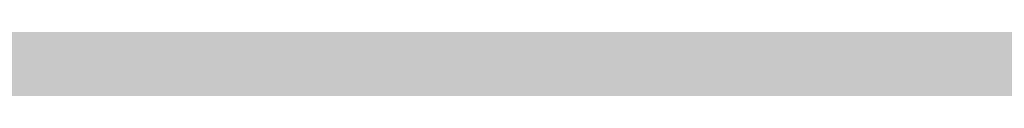
# Model space of a CAD drawing. Units: millimetres. Extents: x 0 to 2267, y 0 to 1823.
# Tile 126 of 256: x 1600.369 to 1605.705, y 1232.332 to 1232.602. Entities that reach past the tile are written whole.
import ezdxf

# ---------------------------------------------------------------- set-up
doc = ezdxf.new("R2010")
doc.units = ezdxf.units.MM
doc.header["$MEASUREMENT"] = 0
doc.layers.add('M-HATC', color=252, linetype='Continuous', lineweight=18)

msp = doc.modelspace()

# ---------------------------------------------------------------- hatches: boundary and pattern name
at = {"layer": 'M-HATC'}
h = msp.add_hatch(color=256, dxfattribs=at)
h.dxf.hatch_style = 1
h.paths.add_polyline_path([(2065.771, 1618.062, 0.236068), (2055.771, 1638.062), (1381.0868, 1638.062, 0.236068), (1371.0868, 1618.062), (1371.0868, 1603.062), (2055.771, 1603.062), (2065.771, 1603.062)])
h.paths.add_polyline_path([(2062.7718, 1550.2964), (2062.7718, 1560.2964), (1374.086, 1560.2964), (1374.086, 1550.2964), (1374.086, 1540.2964), (1384.086, 1540.2964), (1389.086, 1540.2964), (2062.7718, 1540.2964)])
h.paths.add_polyline_path([(1930.9289, 1282.7656), (1505.9289, 1282.7656), (1587.6276, 1235.5968, 0.131652), (1600.1276, 1232.2475), (1836.7302, 1232.2475, 0.131652), (1849.2302, 1235.5968)])
h.paths.add_polyline_path([(1930.9289, 1117.4171), (1905.9289, 1117.4171), (1505.9289, 1117.4171), (1505.9289, 1077.4171), (1930.9289, 1077.4171)])
h = msp.add_hatch(color=256, dxfattribs=at)
h.dxf.hatch_style = 1
h.paths.add_polyline_path([(2055.771, 1603.062), (1381.0868, 1603.062), (1381.0868, 1598.062), (2055.771, 1598.062)])
h.paths.add_polyline_path([(2055.771, 1598.062), (1381.0868, 1598.062), (1381.0868, 1593.062), (2055.771, 1593.062)])
h.paths.add_polyline_path([(2051.3074, 1536.7609), (1385.5504, 1536.7609), (1385.5504, 1526.7609), (1387.5504, 1526.7609), (1388.5366, 1525.0528), (1385.3319, 1521.2335), (1385.3319, 1521.2226), (2050.2542, 1522.7491), (2048.3212, 1525.0528), (2049.3074, 1526.7609), (2051.3074, 1526.7609)])
edge = h.paths.add_edge_path()
edge.add_arc((1847.5345, 1379.1492), 135, 222.603061, 222.890851, ccw=False)
edge.add_line((1748.1663, 1287.7656), (1683.0921, 1287.7656))
edge.add_arc((1583.7239, 1379.1492), 135, 317.109149, 317.396939, ccw=False)
edge.add_arc((1678.9686, 1290.6707), 5, 222.8909, 317.1091, ccw=False)
edge.add_arc((1774.2133, 1379.1492), 135, 222.603061, 222.890851, ccw=False)
edge.add_line((1674.8451, 1287.7656), (1609.7709, 1287.7656))
edge.add_arc((1510.4027, 1379.1492), 135, 317.109149, 317.396939, ccw=False)
edge.add_arc((1605.6474, 1290.6707), 5, 222.8909, 317.1091, ccw=False)
edge.add_arc((1700.8921, 1379.1492), 135, 222.603061, 222.890851, ccw=False)
edge.add_line((1601.5239, 1287.7656), (1536.4497, 1287.7656))
edge.add_arc((1437.0815, 1379.1492), 135, 317.109149, 317.396939, ccw=False)
edge.add_arc((1532.3262, 1290.6707), 5, 222.8909, 317.1091, ccw=False)
edge.add_arc((1627.5709, 1379.1492), 135, 222.603061, 222.890851, ccw=False)
edge.add_line((1528.2027, 1287.7656), (1505.9289, 1287.7656))
edge.add_spline(control_points=[(1505.9289, 1287.7656), (1504.2622, 1287.7656), (1504.2622, 1282.7656), (1505.9289, 1282.7656)], knot_values=[0, 0, 0, 0, 5, 5, 5, 5], degree=3, periodic=0)
edge.add_line((1505.9289, 1282.7656), (1930.9289, 1282.7656))
edge.add_spline(control_points=[(1930.9289, 1282.7656), (1932.5956, 1282.7656), (1932.5956, 1287.7656), (1930.9289, 1287.7656)], knot_values=[0, 0, 0, 0, 5, 5, 5, 5], degree=3, periodic=0)
edge.add_line((1930.9289, 1287.7656), (1903.0557, 1287.7656))
edge.add_arc((1803.6875, 1379.1492), 135, 317.109149, 317.396939, ccw=False)
edge.add_arc((1898.9322, 1290.6707), 5, 222.8909, 317.1091, ccw=False)
edge.add_arc((1994.1769, 1379.1492), 135, 222.603061, 222.890851, ccw=False)
edge.add_line((1894.8087, 1287.7656), (1829.7345, 1287.7656))
edge.add_arc((1730.3663, 1379.1492), 135, 317.109149, 317.396939, ccw=False)
edge.add_arc((1825.611, 1290.6707), 5, 222.8909, 317.1091, ccw=False)
edge.add_arc((1920.8557, 1379.1492), 135, 222.603061, 222.890851, ccw=False)
edge.add_line((1821.4875, 1287.7656), (1756.4133, 1287.7656))
edge.add_arc((1657.0451, 1379.1492), 135, 317.109149, 317.396939, ccw=False)
edge.add_arc((1752.2898, 1290.6707), 5, 222.8909, 317.1091, ccw=False)
edge = h.paths.add_edge_path()
edge.add_spline(control_points=[(1843.4289, 1227.2475), (1845.0956, 1227.2475), (1845.0956, 1232.2475), (1843.4289, 1232.2475)], knot_values=[0, 0, 0, 0, 5, 5, 5, 5], degree=3, periodic=0)
edge.add_line((1843.4289, 1232.2475), (1593.4289, 1232.2475))
edge.add_spline(control_points=[(1593.4289, 1232.2475), (1591.7622, 1232.2475), (1591.7622, 1227.2475), (1593.4289, 1227.2475)], knot_values=[0, 0, 0, 0, 5, 5, 5, 5], degree=3, periodic=0)
edge.add_line((1593.4289, 1227.2475), (1843.4289, 1227.2475))
h.paths.add_polyline_path([(1905.9289, 1127.4171), (1530.9289, 1127.4171, 0.414214), (1520.9289, 1117.4171), (1530.9289, 1117.4171), (1915.9289, 1117.4171, 0.414214)])
edge = h.paths.add_edge_path()
edge.add_arc((1397.0858, 1498.4078), 12.7299, 90.78215, 190.87871, ccw=False)
edge.add_line((1396.912, 1511.1365), (1428.0097, 1511.3488))
edge.add_line((1428.0097, 1511.3488), (1433.0097, 1511.3488))
edge.add_line((1433.0097, 1511.3488), (1434.439, 1511.3488))
edge.add_arc((1419.474, 1498.0804), 20, 41.561, 74.08211)
edge.add_line((1424.9592, 1517.3135), (1399.9351, 1517.2561))
edge.add_spline(control_points=[(1399.9307, 1517.2561), (1399.884, 1517.2131), (1399.8328, 1517.1689), (1399.7774, 1517.1236)], knot_values=[11.567499, 11.567499, 11.567499, 11.567499, 11.814249, 11.814249, 11.814249, 11.814249], degree=3, periodic=0)
edge.add_spline(control_points=[(1399.6328, 1517.0099), (1399.5831, 1516.9721), (1399.5307, 1516.9338), (1399.4759, 1516.8947)], knot_values=[11.167718, 11.167718, 11.167718, 11.167718, 11.365188, 11.365188, 11.365188, 11.365188], degree=3, periodic=0)
edge.add_spline(control_points=[(1399.3398, 1516.8001), (1399.1514, 1516.6719), (1398.9384, 1516.5377), (1398.704, 1516.3994)], knot_values=[10.376405, 10.376405, 10.376405, 10.376405, 11.00994, 11.00994, 11.00994, 11.00994], degree=3, periodic=0)
edge.add_spline(control_points=[(1398.6572, 1516.3719), (1398.5789, 1516.326), (1398.4983, 1516.2797), (1398.4155, 1516.2331)], knot_values=[10.125175, 10.125175, 10.125175, 10.125175, 10.334406, 10.334406, 10.334406, 10.334406], degree=3, periodic=0)
edge.add_spline(control_points=[(1398.2642, 1516.1487), (1398.196, 1516.1111), (1398.1263, 1516.0732), (1398.0555, 1516.0351)], knot_values=[9.832246, 9.832246, 9.832246, 9.832246, 9.999658, 9.999658, 9.999658, 9.999658], degree=3, periodic=0)
edge.add_spline(control_points=[(1397.9987, 1516.0048), (1397.7312, 1515.8621), (1397.446, 1515.7171), (1397.1466, 1515.5714)], knot_values=[9.161808, 9.161808, 9.161808, 9.161808, 9.787769, 9.787769, 9.787769, 9.787769], degree=3, periodic=0)
edge.add_spline(control_points=[(1397.1466, 1515.5714), (1396.8418, 1515.423), (1396.5222, 1515.274), (1396.1914, 1515.1262)], knot_values=[8.524455, 8.524455, 8.524455, 8.524455, 9.161808, 9.161808, 9.161808, 9.161808], degree=3, periodic=0)
edge.add_spline(control_points=[(1396.0777, 1515.0756), (1395.9854, 1515.0348), (1395.8922, 1514.994), (1395.7983, 1514.9534)], knot_values=[8.275193, 8.275193, 8.275193, 8.275193, 8.451726, 8.451726, 8.451726, 8.451726], degree=3, periodic=0)
edge.add_spline(control_points=[(1395.6018, 1514.8691), (1395.4997, 1514.8257), (1395.3968, 1514.7824), (1395.2932, 1514.7394)], knot_values=[7.962917, 7.962917, 7.962917, 7.962917, 8.152764, 8.152764, 8.152764, 8.152764], degree=3, periodic=0)
edge.add_spline(control_points=[(1395.2116, 1514.7057), (1394.8278, 1514.5475), (1394.4345, 1514.3929), (1394.0364, 1514.2442)], knot_values=[7.21254, 7.21254, 7.21254, 7.21254, 7.913148, 7.913148, 7.913148, 7.913148], degree=3, periodic=0)
edge.add_spline(control_points=[(1394.0364, 1514.2442), (1393.7076, 1514.1214), (1393.3754, 1514.0027), (1393.0427, 1513.8895)], knot_values=[6.633733, 6.633733, 6.633733, 6.633733, 7.21254, 7.21254, 7.21254, 7.21254], degree=3, periodic=0)
edge.add_spline(control_points=[(1392.8214, 1513.815), (1392.7198, 1513.7812), (1392.6181, 1513.7479), (1392.5166, 1513.7152)], knot_values=[6.328796, 6.328796, 6.328796, 6.328796, 6.505493, 6.505493, 6.505493, 6.505493], degree=3, periodic=0)
edge.add_spline(control_points=[(1392.5166, 1513.7152), (1392.3187, 1513.6515), (1392.1212, 1513.59), (1391.9244, 1513.531)], knot_values=[5.984605, 5.984605, 5.984605, 5.984605, 6.328796, 6.328796, 6.328796, 6.328796], degree=3, periodic=0)
edge.add_spline(control_points=[(1391.7915, 1513.4915), (1391.3122, 1513.3501), (1390.8384, 1513.2239), (1390.3784, 1513.1171)], knot_values=[5.066697, 5.066697, 5.066697, 5.066697, 5.907055, 5.907055, 5.907055, 5.907055], degree=3, periodic=0)
edge.add_spline(control_points=[(1390.3784, 1513.1171), (1390.1797, 1513.071), (1389.9836, 1513.0284), (1389.7907, 1512.9899)], knot_values=[4.70367, 4.70367, 4.70367, 4.70367, 5.066695, 5.066695, 5.066695, 5.066695], degree=3, periodic=0)
edge.add_spline(control_points=[(1389.422, 1512.9204), (1389.2459, 1512.8892), (1389.0729, 1512.8617), (1388.9036, 1512.8381)], knot_values=[4.130571, 4.130571, 4.130571, 4.130571, 4.469816, 4.469816, 4.469816, 4.469816], degree=3, periodic=0)
edge.add_spline(control_points=[(1388.9036, 1512.8381), (1388.591, 1512.7946), (1388.2911, 1512.7644), (1388.0071, 1512.7494)], knot_values=[3.504031, 3.504031, 3.504031, 3.504031, 4.130571, 4.130571, 4.130571, 4.130571], degree=3, periodic=0)
edge.add_spline(control_points=[(1387.9356, 1512.7459), (1387.8538, 1512.7423), (1387.7733, 1512.74), (1387.6944, 1512.739)], knot_values=[3.268866, 3.268866, 3.268866, 3.268866, 3.451164, 3.451164, 3.451164, 3.451164], degree=3, periodic=0)
edge.add_spline(control_points=[(1387.3351, 1512.7443), (1387.2076, 1512.7499), (1387.0847, 1512.7597), (1386.967, 1512.7739)], knot_values=[2.670686, 2.670686, 2.670686, 2.670686, 2.984, 2.984, 2.984, 2.984], degree=3, periodic=0)
edge.add_spline(control_points=[(1386.8327, 1512.7922), (1386.8209, 1512.7941), (1386.8092, 1512.7959), (1386.7975, 1512.7979)], knot_values=[2.516981, 2.516981, 2.516981, 2.516981, 2.549528, 2.549528, 2.549528, 2.549528], degree=3, periodic=0)
edge.add_spline(control_points=[(1386.4526, 1512.8735), (1386.4257, 1512.881), (1386.3993, 1512.889), (1386.3733, 1512.8972)], knot_values=[2.095869, 2.095869, 2.095869, 2.095869, 2.17941, 2.17941, 2.17941, 2.17941], degree=3, periodic=0)
edge.add_spline(control_points=[(1386.0691, 1513.0189), (1386.0634, 1513.0217), (1386.0577, 1513.0246), (1386.052, 1513.0275)], knot_values=[1.72453, 1.72453, 1.72453, 1.72453, 1.745933, 1.745933, 1.745933, 1.745933], degree=3, periodic=0)
edge.add_arc((1399.474, 1498.0804), 20, 131.82432, 180)
edge.add_arc((1630.3336, 1505.5484), 250.9708, 181.705176, 236.427975)
edge.add_arc((1605.3399, 1483.3044), 218.7822, 238.660829, 243.34961)
edge.add_arc((1647.0911, 1510.3592), 262.8986, 183.129836, 237.853442, ccw=False)
h.paths.add_polyline_path([(1406.5369, 1391.9644, 0.149382), (1491.5506, 1296.4418, -0.129517)], flags=17)
edge = h.paths.add_edge_path()
edge.add_arc((2037.3838, 1498.0804), 20, 0, 48.26587)
edge.add_spline(control_points=[(2050.6973, 1513.0052), (2050.6512, 1512.9847), (2050.6034, 1512.9655), (2050.5539, 1512.9477)], knot_values=[1.835652, 1.835652, 1.835652, 1.835652, 2.000781, 2.000781, 2.000781, 2.000781], degree=3, periodic=0)
edge.add_spline(control_points=[(2050.4616, 1512.9166), (2050.479, 1512.9221), (2050.4963, 1512.9277), (2050.5133, 1512.9335)], knot_values=[2.045477, 2.045477, 2.045477, 2.045477, 2.101389, 2.101389, 2.101389, 2.101389], degree=3, periodic=0)
edge.add_spline(control_points=[(2050.129, 1512.8342), (2050.1984, 1512.8473), (2050.2657, 1512.8623), (2050.3308, 1512.8792)], knot_values=[2.237629, 2.237629, 2.237629, 2.237629, 2.435841, 2.435841, 2.435841, 2.435841], degree=3, periodic=0)
edge.add_spline(control_points=[(2050.0946, 1512.8278), (2050.1061, 1512.8299), (2050.1176, 1512.832), (2050.129, 1512.8342)], knot_values=[2.435841, 2.435841, 2.435841, 2.435841, 2.468321, 2.468321, 2.468321, 2.468321], degree=3, periodic=0)
edge.add_spline(control_points=[(2049.7843, 1512.7851), (2049.8552, 1512.7922), (2049.9243, 1512.8008), (2049.9917, 1512.8109)], knot_values=[2.563852, 2.563852, 2.563852, 2.563852, 2.748541, 2.748541, 2.748541, 2.748541], degree=3, periodic=0)
edge.add_spline(control_points=[(2049.4052, 1512.7617), (2049.5364, 1512.7653), (2049.6629, 1512.773), (2049.7843, 1512.7851)], knot_values=[2.748541, 2.748541, 2.748541, 2.748541, 3.064882, 3.064882, 3.064882, 3.064882], degree=3, periodic=0)
edge.add_spline(control_points=[(2049.1698, 1512.7597), (2049.2336, 1512.7591), (2049.2965, 1512.7594), (2049.3584, 1512.7606)], knot_values=[3.102309, 3.102309, 3.102309, 3.102309, 3.2503, 3.2503, 3.2503, 3.2503], degree=3, periodic=0)
edge.add_spline(control_points=[(2048.8573, 1512.7691), (2048.9638, 1512.7638), (2049.068, 1512.7606), (2049.1698, 1512.7597)], knot_values=[3.2503, 3.2503, 3.2503, 3.2503, 3.486069, 3.486069, 3.486069, 3.486069], degree=3, periodic=0)
edge.add_spline(control_points=[(2048.6924, 1512.7789), (2048.3729, 1512.8009), (2048.0345, 1512.8411), (2047.6817, 1512.897)], knot_values=[3.606429, 3.606429, 3.606429, 3.606429, 4.2989, 4.2989, 4.2989, 4.2989], degree=3, periodic=0)
edge.add_spline(control_points=[(2047.6817, 1512.897), (2047.5458, 1512.9185), (2047.4077, 1512.9424), (2047.2678, 1512.9685)], knot_values=[4.2989, 4.2989, 4.2989, 4.2989, 4.565769, 4.565769, 4.565769, 4.565769], degree=3, periodic=0)
edge.add_spline(control_points=[(2047.2678, 1512.9685), (2047.1449, 1512.9914), (2047.0207, 1513.016), (2046.8951, 1513.0422)], knot_values=[4.565769, 4.565769, 4.565769, 4.565769, 4.799971, 4.799971, 4.799971, 4.799971], degree=3, periodic=0)
edge.add_spline(control_points=[(2046.8951, 1513.0422), (2046.5286, 1513.1188), (2046.1513, 1513.209), (2045.7676, 1513.3107)], knot_values=[4.799971, 4.799971, 4.799971, 4.799971, 5.483718, 5.483718, 5.483718, 5.483718], degree=3, periodic=0)
edge.add_spline(control_points=[(2045.7676, 1513.3107), (2045.3724, 1513.4154), (2044.9704, 1513.5322), (2044.5662, 1513.6588)], knot_values=[5.483718, 5.483718, 5.483718, 5.483718, 6.187866, 6.187866, 6.187866, 6.187866], degree=3, periodic=0)
edge.add_spline(control_points=[(2044.5662, 1513.6588), (2044.4149, 1513.7061), (2044.2633, 1513.7549), (2044.1116, 1513.8048)], knot_values=[6.187866, 6.187866, 6.187866, 6.187866, 6.451551, 6.451551, 6.451551, 6.451551], degree=3, periodic=0)
edge.add_spline(control_points=[(2044.1116, 1513.8048), (2043.9967, 1513.8427), (2043.8817, 1513.8813), (2043.7668, 1513.9205)], knot_values=[6.451551, 6.451551, 6.451551, 6.451551, 6.651434, 6.651434, 6.651434, 6.651434], degree=3, periodic=0)
edge.add_spline(control_points=[(2043.7668, 1513.9205), (2043.3716, 1514.0554), (2042.9774, 1514.1979), (2042.5886, 1514.3458)], knot_values=[6.651434, 6.651434, 6.651434, 6.651434, 7.338879, 7.338879, 7.338879, 7.338879], degree=3, periodic=0)
edge.add_spline(control_points=[(2042.5886, 1514.3458), (2042.1643, 1514.5071), (2041.7465, 1514.6749), (2041.3409, 1514.846)], knot_values=[7.338879, 7.338879, 7.338879, 7.338879, 8.089209, 8.089209, 8.089209, 8.089209], degree=3, periodic=0)
edge.add_spline(control_points=[(2041.3409, 1514.846), (2041.1028, 1514.9465), (2040.869, 1515.0481), (2040.6405, 1515.1502)], knot_values=[8.089209, 8.089209, 8.089209, 8.089209, 8.529587, 8.529587, 8.529587, 8.529587], degree=3, periodic=0)
edge.add_spline(control_points=[(2040.51, 1515.2089), (2040.0824, 1515.4022), (2039.6747, 1515.5971), (2039.295, 1515.7894)], knot_values=[8.613818, 8.613818, 8.613818, 8.613818, 9.44571, 9.44571, 9.44571, 9.44571], degree=3, periodic=0)
edge.add_spline(control_points=[(2039.295, 1515.7894), (2039.0618, 1515.9075), (2038.8391, 1516.0246), (2038.6288, 1516.1398)], knot_values=[9.44571, 9.44571, 9.44571, 9.44571, 9.956404, 9.956404, 9.956404, 9.956404], degree=3, periodic=0)
edge.add_spline(control_points=[(2038.6288, 1516.1398), (2038.5187, 1516.2001), (2038.4121, 1516.2598), (2038.309, 1516.3189)], knot_values=[9.956404, 9.956404, 9.956404, 9.956404, 10.223542, 10.223542, 10.223542, 10.223542], degree=3, periodic=0)
edge.add_spline(control_points=[(2038.309, 1516.3189), (2038.2138, 1516.3735), (2038.1216, 1516.4276), (2038.0328, 1516.481)], knot_values=[10.223542, 10.223542, 10.223542, 10.223542, 10.47051, 10.47051, 10.47051, 10.47051], degree=3, periodic=0)
edge.add_spline(control_points=[(2038.0328, 1516.481), (2037.7855, 1516.6296), (2037.5639, 1516.773), (2037.3722, 1516.909)], knot_values=[10.47051, 10.47051, 10.47051, 10.47051, 11.15767, 11.15767, 11.15767, 11.15767], degree=3, periodic=0)
edge.add_spline(control_points=[(2037.3722, 1516.909), (2037.2789, 1516.9752), (2037.1927, 1517.0396), (2037.1142, 1517.102)], knot_values=[11.15767, 11.15767, 11.15767, 11.15767, 11.49227, 11.49227, 11.49227, 11.49227], degree=3, periodic=0)
edge.add_spline(control_points=[(2036.8564, 1517.3259), (2036.9148, 1517.2692), (2036.9814, 1517.2103), (2037.0557, 1517.1492)], knot_values=[11.577341, 11.577341, 11.577341, 11.577341, 11.91035, 11.91035, 11.91035, 11.91035], degree=3, periodic=0)
edge.add_spline(control_points=[(2036.8074, 1517.3748), (2036.823, 1517.3587), (2036.8393, 1517.3424), (2036.8564, 1517.3259)], knot_values=[11.91035, 11.91035, 11.91035, 11.91035, 12.007402, 12.007402, 12.007402, 12.007402], degree=3, periodic=0)
edge.add_spline(control_points=[(2036.7017, 1517.494), (2036.7104, 1517.483), (2036.7196, 1517.4719), (2036.7291, 1517.4606)], knot_values=[12.184155, 12.184155, 12.184155, 12.184155, 12.255409, 12.255409, 12.255409, 12.255409], degree=3, periodic=0)
edge.add_spline(control_points=[(2036.6159, 1517.6205), (2036.62, 1517.613), (2036.6243, 1517.6055), (2036.6289, 1517.5979)], knot_values=[12.487913, 12.487913, 12.487913, 12.487913, 12.541035, 12.541035, 12.541035, 12.541035], degree=3, periodic=0)
edge.add_spline(control_points=[(2036.5635, 1517.786), (2036.5637, 1517.7794), (2036.5642, 1517.7726), (2036.565, 1517.7658)], knot_values=[12.911761, 12.911761, 12.911761, 12.911761, 12.968286, 12.968286, 12.968286, 12.968286], degree=3, periodic=0)
edge.add_spline(control_points=[(2036.6166, 1517.9304), (2036.6125, 1517.9259), (2036.6086, 1517.9212), (2036.6049, 1517.9165)], knot_values=[13.382527, 13.382527, 13.382527, 13.382527, 13.433791, 13.433791, 13.433791, 13.433791], degree=3, periodic=0)
edge.add_spline(control_points=[(2036.749, 1518.017), (2036.7361, 1518.0116), (2036.7239, 1518.006), (2036.7124, 1518.0002)], knot_values=[13.726299, 13.726299, 13.726299, 13.726299, 13.809928, 13.809928, 13.809928, 13.809928], degree=3, periodic=0)
edge.add_spline(control_points=[(2036.8604, 1518.0528), (2036.8386, 1518.0474), (2036.8181, 1518.0416), (2036.7988, 1518.0353)], knot_values=[13.910887, 13.910887, 13.910887, 13.910887, 14.02153, 14.02153, 14.02153, 14.02153], degree=3, periodic=0)
edge.add_line((2036.9639, 1518.0804), (2032.3838, 1518.0804))
edge.add_line((2032.3838, 1518.0804), (2027.3838, 1518.0804))
edge.add_line((2027.3838, 1518.0804), (2022.3838, 1518.0804))
edge.add_line((2022.3838, 1518.0804), (2017.3838, 1518.0804))
edge.add_arc((2017.3838, 1498.0804), 20, 90, 138.439)
edge.add_line((2002.4188, 1511.3488), (2003.8481, 1511.3488))
edge.add_line((2003.8481, 1511.3488), (2008.8481, 1511.3488))
edge.add_line((2008.8481, 1511.3488), (2039.772, 1511.1377))
edge.add_arc((2039.772, 1498.4078), 12.7299, -10.87871, 90, ccw=False)
edge.add_arc((1789.7668, 1510.3592), 262.8986, 302.146558, 356.870164, ccw=False)
edge.add_arc((1831.5179, 1483.3044), 218.7822, 296.65039, 301.339171)
edge.add_arc((1806.5242, 1505.5484), 250.9708, 303.572025, 358.294824)
h.paths.add_polyline_path([(2030.321, 1391.9644, -0.129517), (1945.3072, 1296.4418, 0.149382)], flags=17)
edge = h.paths.add_edge_path()
edge.add_spline(control_points=[(2037.2464, 1518.0821), (2037.2898, 1518.081), (2037.3355, 1518.0804), (2037.3838, 1518.0804)], knot_values=[0.000012, 0.000012, 0.000012, 0.000012, 0.144754, 0.144754, 0.144754, 0.144754], degree=3, periodic=0)
edge.add_line((2037.3357, 1518.0804), (2037.0096, 1518.0804))
edge.add_spline(control_points=[(2037.0096, 1518.0804), (2036.9822, 1518.0768), (2036.956, 1518.0727), (2036.9312, 1518.0681)], knot_values=[14.13465, 14.13465, 14.13465, 14.13465, 14.247197, 14.247197, 14.247197, 14.247197], degree=3, periodic=0)
edge.add_spline(control_points=[(2036.9312, 1518.0681), (2036.9276, 1518.0674), (2036.9241, 1518.0667), (2036.9205, 1518.0661)], knot_values=[14.118315, 14.118315, 14.118315, 14.118315, 14.13465, 14.13465, 14.13465, 14.13465], degree=3, periodic=0)
edge.add_spline(control_points=[(2036.9205, 1518.0661), (2036.9118, 1518.0644), (2036.9032, 1518.0626), (2036.8948, 1518.0608)], knot_values=[14.078086, 14.078086, 14.078086, 14.078086, 14.118315, 14.118315, 14.118315, 14.118315], degree=3, periodic=0)
edge.add_spline(control_points=[(2036.8948, 1518.0608), (2036.883, 1518.0583), (2036.8716, 1518.0556), (2036.8604, 1518.0528)], knot_values=[14.02153, 14.02153, 14.02153, 14.02153, 14.078086, 14.078086, 14.078086, 14.078086], degree=3, periodic=0)
edge.add_spline(control_points=[(2036.8604, 1518.0528), (2036.8386, 1518.0474), (2036.8181, 1518.0416), (2036.7988, 1518.0353)], knot_values=[13.910887, 13.910887, 13.910887, 13.910887, 14.02153, 14.02153, 14.02153, 14.02153], degree=3, periodic=0)
edge.add_spline(control_points=[(2036.7988, 1518.0353), (2036.7981, 1518.035), (2036.7974, 1518.0348), (2036.7967, 1518.0346)], knot_values=[13.906906, 13.906906, 13.906906, 13.906906, 13.910887, 13.910887, 13.910887, 13.910887], degree=3, periodic=0)
edge.add_spline(control_points=[(2036.7967, 1518.0346), (2036.7882, 1518.0318), (2036.7799, 1518.0289), (2036.7719, 1518.0259)], knot_values=[13.857826, 13.857826, 13.857826, 13.857826, 13.906906, 13.906906, 13.906906, 13.906906], degree=3, periodic=0)
edge.add_spline(control_points=[(2036.7719, 1518.0259), (2036.764, 1518.023), (2036.7564, 1518.02), (2036.749, 1518.017)], knot_values=[13.809928, 13.809928, 13.809928, 13.809928, 13.857826, 13.857826, 13.857826, 13.857826], degree=3, periodic=0)
edge.add_spline(control_points=[(2036.749, 1518.017), (2036.7361, 1518.0116), (2036.7239, 1518.006), (2036.7124, 1518.0002)], knot_values=[13.726299, 13.726299, 13.726299, 13.726299, 13.809928, 13.809928, 13.809928, 13.809928], degree=3, periodic=0)
edge.add_spline(control_points=[(2036.7124, 1518.0002), (2036.7121, 1518), (2036.7118, 1517.9999), (2036.7115, 1517.9997)], knot_values=[13.723993, 13.723993, 13.723993, 13.723993, 13.726299, 13.726299, 13.726299, 13.726299], degree=3, periodic=0)
edge.add_spline(control_points=[(2036.7115, 1517.9997), (2036.7063, 1517.9971), (2036.7013, 1517.9944), (2036.6965, 1517.9917)], knot_values=[13.686536, 13.686536, 13.686536, 13.686536, 13.723993, 13.723993, 13.723993, 13.723993], degree=3, periodic=0)
edge.add_spline(control_points=[(2036.6965, 1517.9917), (2036.6919, 1517.9891), (2036.6874, 1517.9865), (2036.6831, 1517.9839)], knot_values=[13.651251, 13.651251, 13.651251, 13.651251, 13.686536, 13.686536, 13.686536, 13.686536], degree=3, periodic=0)
edge.add_spline(control_points=[(2036.6831, 1517.9839), (2036.6764, 1517.9798), (2036.67, 1517.9757), (2036.6639, 1517.9714)], knot_values=[13.596804, 13.596804, 13.596804, 13.596804, 13.651251, 13.651251, 13.651251, 13.651251], degree=3, periodic=0)
edge.add_spline(control_points=[(2036.6639, 1517.9714), (2036.6636, 1517.9712), (2036.6633, 1517.9709), (2036.6629, 1517.9707)], knot_values=[13.593956, 13.593956, 13.593956, 13.593956, 13.596804, 13.596804, 13.596804, 13.596804], degree=3, periodic=0)
edge.add_spline(control_points=[(2036.6629, 1517.9707), (2036.6603, 1517.9689), (2036.6577, 1517.967), (2036.6552, 1517.9651)], knot_values=[13.570322, 13.570322, 13.570322, 13.570322, 13.593956, 13.593956, 13.593956, 13.593956], degree=3, periodic=0)
edge.add_spline(control_points=[(2036.6552, 1517.9651), (2036.6525, 1517.9631), (2036.6499, 1517.9611), (2036.6474, 1517.9591)], knot_values=[13.545477, 13.545477, 13.545477, 13.545477, 13.570322, 13.570322, 13.570322, 13.570322], degree=3, periodic=0)
edge.add_spline(control_points=[(2036.6474, 1517.9591), (2036.6472, 1517.9589), (2036.6471, 1517.9588), (2036.6469, 1517.9587)], knot_values=[13.543931, 13.543931, 13.543931, 13.543931, 13.545477, 13.545477, 13.545477, 13.545477], degree=3, periodic=0)
edge.add_spline(control_points=[(2036.6469, 1517.9587), (2036.6412, 1517.9541), (2036.6358, 1517.9494), (2036.6307, 1517.9447)], knot_values=[13.488237, 13.488237, 13.488237, 13.488237, 13.543931, 13.543931, 13.543931, 13.543931], degree=3, periodic=0)
edge.add_spline(control_points=[(2036.6307, 1517.9447), (2036.6282, 1517.9423), (2036.6257, 1517.9399), (2036.6233, 1517.9374)], knot_values=[13.460307, 13.460307, 13.460307, 13.460307, 13.488237, 13.488237, 13.488237, 13.488237], degree=3, periodic=0)
edge.add_spline(control_points=[(2036.6233, 1517.9374), (2036.6215, 1517.9356), (2036.6198, 1517.9338), (2036.6181, 1517.932)], knot_values=[13.439712, 13.439712, 13.439712, 13.439712, 13.460307, 13.460307, 13.460307, 13.460307], degree=3, periodic=0)
edge.add_spline(control_points=[(2036.6181, 1517.932), (2036.6176, 1517.9315), (2036.6171, 1517.9309), (2036.6166, 1517.9304)], knot_values=[13.433791, 13.433791, 13.433791, 13.433791, 13.439712, 13.439712, 13.439712, 13.439712], degree=3, periodic=0)
edge.add_spline(control_points=[(2036.6166, 1517.9304), (2036.6125, 1517.9259), (2036.6086, 1517.9212), (2036.6049, 1517.9165)], knot_values=[13.382527, 13.382527, 13.382527, 13.382527, 13.433791, 13.433791, 13.433791, 13.433791], degree=3, periodic=0)
edge.add_spline(control_points=[(2036.6049, 1517.9165), (2036.6026, 1517.9135), (2036.6004, 1517.9104), (2036.5982, 1517.9074)], knot_values=[13.350017, 13.350017, 13.350017, 13.350017, 13.382527, 13.382527, 13.382527, 13.382527], degree=3, periodic=0)
edge.add_spline(control_points=[(2036.5982, 1517.9074), (2036.5972, 1517.9059), (2036.5962, 1517.9043), (2036.5952, 1517.9028)], knot_values=[13.333922, 13.333922, 13.333922, 13.333922, 13.350017, 13.350017, 13.350017, 13.350017], degree=3, periodic=0)
edge.add_spline(control_points=[(2036.5952, 1517.9028), (2036.5945, 1517.9018), (2036.5939, 1517.9009), (2036.5933, 1517.8999)], knot_values=[13.323828, 13.323828, 13.323828, 13.323828, 13.333922, 13.333922, 13.333922, 13.333922], degree=3, periodic=0)
edge.add_spline(control_points=[(2036.5933, 1517.8999), (2036.5905, 1517.8955), (2036.5879, 1517.8909), (2036.5855, 1517.8864)], knot_values=[13.277545, 13.277545, 13.277545, 13.277545, 13.323828, 13.323828, 13.323828, 13.323828], degree=3, periodic=0)
edge.add_spline(control_points=[(2036.5855, 1517.8864), (2036.5836, 1517.8827), (2036.5817, 1517.8789), (2036.5801, 1517.8751)], knot_values=[13.240119, 13.240119, 13.240119, 13.240119, 13.277545, 13.277545, 13.277545, 13.277545], degree=3, periodic=0)
edge.add_spline(control_points=[(2036.5801, 1517.8751), (2036.5795, 1517.8739), (2036.579, 1517.8727), (2036.5785, 1517.8715)], knot_values=[13.228211, 13.228211, 13.228211, 13.228211, 13.240119, 13.240119, 13.240119, 13.240119], degree=3, periodic=0)
edge.add_spline(control_points=[(2036.5785, 1517.8715), (2036.578, 1517.8702), (2036.5774, 1517.869), (2036.5769, 1517.8677)], knot_values=[13.215717, 13.215717, 13.215717, 13.215717, 13.228211, 13.228211, 13.228211, 13.228211], degree=3, periodic=0)
edge.add_spline(control_points=[(2036.5769, 1517.8677), (2036.5755, 1517.864), (2036.5741, 1517.8603), (2036.5729, 1517.8565)], knot_values=[13.179847, 13.179847, 13.179847, 13.179847, 13.215717, 13.215717, 13.215717, 13.215717], degree=3, periodic=0)
edge.add_spline(control_points=[(2036.5729, 1517.8565), (2036.5713, 1517.8515), (2036.5699, 1517.8464), (2036.5687, 1517.8413)], knot_values=[13.132017, 13.132017, 13.132017, 13.132017, 13.179847, 13.179847, 13.179847, 13.179847], degree=3, periodic=0)
edge.add_spline(control_points=[(2036.5687, 1517.8413), (2036.5684, 1517.8402), (2036.5682, 1517.8392), (2036.568, 1517.8382)], knot_values=[13.122482, 13.122482, 13.122482, 13.122482, 13.132017, 13.132017, 13.132017, 13.132017], degree=3, periodic=0)
edge.add_spline(control_points=[(2036.568, 1517.8382), (2036.5676, 1517.8363), (2036.5672, 1517.8345), (2036.5669, 1517.8327)], knot_values=[13.105592, 13.105592, 13.105592, 13.105592, 13.122482, 13.122482, 13.122482, 13.122482], degree=3, periodic=0)
edge.add_spline(control_points=[(2036.5669, 1517.8327), (2036.5662, 1517.8292), (2036.5657, 1517.8257), (2036.5652, 1517.8222)], knot_values=[13.074063, 13.074063, 13.074063, 13.074063, 13.105592, 13.105592, 13.105592, 13.105592], degree=3, periodic=0)
edge.add_spline(control_points=[(2036.5652, 1517.8222), (2036.5652, 1517.8222), (2036.5652, 1517.8222), (2036.5652, 1517.8222)], knot_values=[13.074043, 13.074043, 13.074043, 13.074043, 13.074063, 13.074063, 13.074063, 13.074063], degree=3, periodic=0)
edge.add_spline(control_points=[(2036.5652, 1517.8222), (2036.5644, 1517.8164), (2036.5639, 1517.8106), (2036.5636, 1517.8046)], knot_values=[13.021884, 13.021884, 13.021884, 13.021884, 13.074043, 13.074043, 13.074043, 13.074043], degree=3, periodic=0)
edge.add_spline(control_points=[(2036.5636, 1517.8046), (2036.5636, 1517.804), (2036.5636, 1517.8034), (2036.5635, 1517.8028)], knot_values=[13.01674, 13.01674, 13.01674, 13.01674, 13.021884, 13.021884, 13.021884, 13.021884], degree=3, periodic=0)
edge.add_spline(control_points=[(2036.5635, 1517.8028), (2036.5634, 1517.8005), (2036.5634, 1517.7982), (2036.5634, 1517.7958)], knot_values=[12.996438, 12.996438, 12.996438, 12.996438, 13.01674, 13.01674, 13.01674, 13.01674], degree=3, periodic=0)
edge.add_spline(control_points=[(2036.5634, 1517.7958), (2036.5633, 1517.7926), (2036.5634, 1517.7893), (2036.5635, 1517.786)], knot_values=[12.968286, 12.968286, 12.968286, 12.968286, 12.996438, 12.996438, 12.996438, 12.996438], degree=3, periodic=0)
edge.add_spline(control_points=[(2036.5635, 1517.786), (2036.5637, 1517.7794), (2036.5642, 1517.7726), (2036.565, 1517.7658)], knot_values=[12.911761, 12.911761, 12.911761, 12.911761, 12.968286, 12.968286, 12.968286, 12.968286], degree=3, periodic=0)
edge.add_spline(control_points=[(2036.565, 1517.7658), (2036.565, 1517.7657), (2036.565, 1517.7656), (2036.565, 1517.7656)], knot_values=[12.911017, 12.911017, 12.911017, 12.911017, 12.911761, 12.911761, 12.911761, 12.911761], degree=3, periodic=0)
edge.add_spline(control_points=[(2036.565, 1517.7656), (2036.5654, 1517.7625), (2036.5658, 1517.7593), (2036.5663, 1517.7562)], knot_values=[12.88528, 12.88528, 12.88528, 12.88528, 12.911017, 12.911017, 12.911017, 12.911017], degree=3, periodic=0)
edge.add_spline(control_points=[(2036.5663, 1517.7562), (2036.5667, 1517.7534), (2036.5672, 1517.7506), (2036.5677, 1517.7478)], knot_values=[12.862519, 12.862519, 12.862519, 12.862519, 12.88528, 12.88528, 12.88528, 12.88528], degree=3, periodic=0)
edge.add_spline(control_points=[(2036.5677, 1517.7478), (2036.5678, 1517.7474), (2036.5679, 1517.7469), (2036.568, 1517.7465)], knot_values=[12.858885, 12.858885, 12.858885, 12.858885, 12.862519, 12.862519, 12.862519, 12.862519], degree=3, periodic=0)
edge.add_spline(control_points=[(2036.568, 1517.7465), (2036.5692, 1517.7399), (2036.5707, 1517.7332), (2036.5724, 1517.7264)], knot_values=[12.8053, 12.8053, 12.8053, 12.8053, 12.858885, 12.858885, 12.858885, 12.858885], degree=3, periodic=0)
edge.add_spline(control_points=[(2036.5724, 1517.7264), (2036.5734, 1517.7226), (2036.5745, 1517.7187), (2036.5756, 1517.7149)], knot_values=[12.775176, 12.775176, 12.775176, 12.775176, 12.8053, 12.8053, 12.8053, 12.8053], degree=3, periodic=0)
edge.add_spline(control_points=[(2036.5756, 1517.7149), (2036.5763, 1517.7125), (2036.577, 1517.7102), (2036.5778, 1517.7078)], knot_values=[12.756759, 12.756759, 12.756759, 12.756759, 12.775176, 12.775176, 12.775176, 12.775176], degree=3, periodic=0)
edge.add_spline(control_points=[(2036.5778, 1517.7078), (2036.5781, 1517.7067), (2036.5784, 1517.7057), (2036.5787, 1517.7047)], knot_values=[12.748742, 12.748742, 12.748742, 12.748742, 12.756759, 12.756759, 12.756759, 12.756759], degree=3, periodic=0)
edge.add_spline(control_points=[(2036.5787, 1517.7047), (2036.5808, 1517.6983), (2036.5831, 1517.6919), (2036.5856, 1517.6854)], knot_values=[12.69959, 12.69959, 12.69959, 12.69959, 12.748742, 12.748742, 12.748742, 12.748742], degree=3, periodic=0)
edge.add_spline(control_points=[(2036.5856, 1517.6854), (2036.5876, 1517.68), (2036.5898, 1517.6746), (2036.5921, 1517.6692)], knot_values=[12.659038, 12.659038, 12.659038, 12.659038, 12.69959, 12.69959, 12.69959, 12.69959], degree=3, periodic=0)
edge.add_spline(control_points=[(2036.5921, 1517.6692), (2036.594, 1517.6648), (2036.5959, 1517.6605), (2036.5979, 1517.6561)], knot_values=[12.626806, 12.626806, 12.626806, 12.626806, 12.659038, 12.659038, 12.659038, 12.659038], degree=3, periodic=0)
edge.add_spline(control_points=[(2036.5979, 1517.6561), (2036.5984, 1517.6551), (2036.5989, 1517.6541), (2036.5993, 1517.6531)], knot_values=[12.619394, 12.619394, 12.619394, 12.619394, 12.626806, 12.626806, 12.626806, 12.626806], degree=3, periodic=0)
edge.add_spline(control_points=[(2036.5993, 1517.6531), (2036.6043, 1517.6424), (2036.6099, 1517.6315), (2036.6159, 1517.6205)], knot_values=[12.541039, 12.541039, 12.541039, 12.541039, 12.619394, 12.619394, 12.619394, 12.619394], degree=3, periodic=0)
edge.add_spline(control_points=[(2036.6159, 1517.6205), (2036.6159, 1517.6205), (2036.6159, 1517.6205), (2036.6159, 1517.6205)], knot_values=[12.541035, 12.541035, 12.541035, 12.541035, 12.541039, 12.541039, 12.541039, 12.541039], degree=3, periodic=0)
edge.add_spline(control_points=[(2036.6159, 1517.6205), (2036.62, 1517.613), (2036.6243, 1517.6055), (2036.6289, 1517.5979)], knot_values=[12.487913, 12.487913, 12.487913, 12.487913, 12.541035, 12.541035, 12.541035, 12.541035], degree=3, periodic=0)
edge.add_spline(control_points=[(2036.6289, 1517.5979), (2036.6326, 1517.5916), (2036.6365, 1517.5853), (2036.6406, 1517.5789)], knot_values=[12.443982, 12.443982, 12.443982, 12.443982, 12.487913, 12.487913, 12.487913, 12.487913], degree=3, periodic=0)
edge.add_spline(control_points=[(2036.6406, 1517.5789), (2036.6414, 1517.5776), (2036.6423, 1517.5763), (2036.6431, 1517.5749)], knot_values=[12.434996, 12.434996, 12.434996, 12.434996, 12.443982, 12.443982, 12.443982, 12.443982], degree=3, periodic=0)
edge.add_spline(control_points=[(2036.6431, 1517.5749), (2036.6531, 1517.5596), (2036.6639, 1517.5439), (2036.6756, 1517.528)], knot_values=[12.329647, 12.329647, 12.329647, 12.329647, 12.434996, 12.434996, 12.434996, 12.434996], degree=3, periodic=0)
edge.add_spline(control_points=[(2036.6756, 1517.528), (2036.6839, 1517.5168), (2036.6925, 1517.5055), (2036.7017, 1517.494)], knot_values=[12.255409, 12.255409, 12.255409, 12.255409, 12.329647, 12.329647, 12.329647, 12.329647], degree=3, periodic=0)
edge.add_spline(control_points=[(2036.7017, 1517.494), (2036.7104, 1517.483), (2036.7196, 1517.4719), (2036.7291, 1517.4606)], knot_values=[12.184155, 12.184155, 12.184155, 12.184155, 12.255409, 12.255409, 12.255409, 12.255409], degree=3, periodic=0)
edge.add_spline(control_points=[(2036.7291, 1517.4606), (2036.7436, 1517.4435), (2036.759, 1517.4262), (2036.7753, 1517.4085)], knot_values=[12.075961, 12.075961, 12.075961, 12.075961, 12.184155, 12.184155, 12.184155, 12.184155], degree=3, periodic=0)
edge.add_spline(control_points=[(2036.7753, 1517.4085), (2036.7763, 1517.4075), (2036.7773, 1517.4064), (2036.7783, 1517.4054)], knot_values=[12.069502, 12.069502, 12.069502, 12.069502, 12.075961, 12.075961, 12.075961, 12.075961], degree=3, periodic=0)
edge.add_spline(control_points=[(2036.7783, 1517.4054), (2036.7877, 1517.3953), (2036.7974, 1517.385), (2036.8074, 1517.3748)], knot_values=[12.007402, 12.007402, 12.007402, 12.007402, 12.069502, 12.069502, 12.069502, 12.069502], degree=3, periodic=0)
edge.add_spline(control_points=[(2036.8074, 1517.3748), (2036.823, 1517.3587), (2036.8393, 1517.3424), (2036.8564, 1517.3259)], knot_values=[11.91035, 11.91035, 11.91035, 11.91035, 12.007402, 12.007402, 12.007402, 12.007402], degree=3, periodic=0)
edge.add_spline(control_points=[(2036.8564, 1517.3259), (2036.9148, 1517.2692), (2036.9814, 1517.2103), (2037.0557, 1517.1492)], knot_values=[11.577341, 11.577341, 11.577341, 11.577341, 11.91035, 11.91035, 11.91035, 11.91035], degree=3, periodic=0)
edge.add_spline(control_points=[(2037.0557, 1517.1492), (2037.0747, 1517.1336), (2037.0942, 1517.1179), (2037.1142, 1517.102)], knot_values=[11.49227, 11.49227, 11.49227, 11.49227, 11.577341, 11.577341, 11.577341, 11.577341], degree=3, periodic=0)
edge.add_spline(control_points=[(2037.1142, 1517.102), (2037.1927, 1517.0396), (2037.2789, 1516.9752), (2037.3722, 1516.909)], knot_values=[11.15767, 11.15767, 11.15767, 11.15767, 11.49227, 11.49227, 11.49227, 11.49227], degree=3, periodic=0)
edge.add_spline(control_points=[(2037.3722, 1516.909), (2037.5639, 1516.773), (2037.7855, 1516.6296), (2038.0328, 1516.481)], knot_values=[10.47051, 10.47051, 10.47051, 10.47051, 11.15767, 11.15767, 11.15767, 11.15767], degree=3, periodic=0)
edge.add_spline(control_points=[(2038.0328, 1516.481), (2038.1216, 1516.4276), (2038.2138, 1516.3735), (2038.309, 1516.3189)], knot_values=[10.223542, 10.223542, 10.223542, 10.223542, 10.47051, 10.47051, 10.47051, 10.47051], degree=3, periodic=0)
edge.add_spline(control_points=[(2038.309, 1516.3189), (2038.4121, 1516.2598), (2038.5187, 1516.2001), (2038.6288, 1516.1398)], knot_values=[9.956404, 9.956404, 9.956404, 9.956404, 10.223542, 10.223542, 10.223542, 10.223542], degree=3, periodic=0)
edge.add_spline(control_points=[(2038.6288, 1516.1398), (2038.8391, 1516.0246), (2039.0618, 1515.9075), (2039.295, 1515.7894)], knot_values=[9.44571, 9.44571, 9.44571, 9.44571, 9.956404, 9.956404, 9.956404, 9.956404], degree=3, periodic=0)
edge.add_spline(control_points=[(2039.295, 1515.7894), (2039.6747, 1515.5971), (2040.0824, 1515.4022), (2040.51, 1515.2089)], knot_values=[8.613818, 8.613818, 8.613818, 8.613818, 9.44571, 9.44571, 9.44571, 9.44571], degree=3, periodic=0)
edge.add_spline(control_points=[(2040.51, 1515.2089), (2040.5533, 1515.1893), (2040.5968, 1515.1697), (2040.6405, 1515.1502)], knot_values=[8.529587, 8.529587, 8.529587, 8.529587, 8.613818, 8.613818, 8.613818, 8.613818], degree=3, periodic=0)
edge.add_spline(control_points=[(2040.6405, 1515.1502), (2040.869, 1515.0481), (2041.1028, 1514.9465), (2041.3409, 1514.846)], knot_values=[8.089209, 8.089209, 8.089209, 8.089209, 8.529587, 8.529587, 8.529587, 8.529587], degree=3, periodic=0)
edge.add_spline(control_points=[(2041.3409, 1514.846), (2041.7465, 1514.6749), (2042.1643, 1514.5071), (2042.5886, 1514.3458)], knot_values=[7.338879, 7.338879, 7.338879, 7.338879, 8.089209, 8.089209, 8.089209, 8.089209], degree=3, periodic=0)
edge.add_spline(control_points=[(2042.5886, 1514.3458), (2042.9774, 1514.1979), (2043.3716, 1514.0554), (2043.7668, 1513.9205)], knot_values=[6.651434, 6.651434, 6.651434, 6.651434, 7.338879, 7.338879, 7.338879, 7.338879], degree=3, periodic=0)
edge.add_spline(control_points=[(2043.7668, 1513.9205), (2043.8817, 1513.8813), (2043.9967, 1513.8427), (2044.1116, 1513.8048)], knot_values=[6.451551, 6.451551, 6.451551, 6.451551, 6.651434, 6.651434, 6.651434, 6.651434], degree=3, periodic=0)
edge.add_spline(control_points=[(2044.1116, 1513.8048), (2044.2633, 1513.7549), (2044.4149, 1513.7061), (2044.5662, 1513.6588)], knot_values=[6.187866, 6.187866, 6.187866, 6.187866, 6.451551, 6.451551, 6.451551, 6.451551], degree=3, periodic=0)
edge.add_spline(control_points=[(2044.5662, 1513.6588), (2044.9704, 1513.5322), (2045.3724, 1513.4154), (2045.7676, 1513.3107)], knot_values=[5.483718, 5.483718, 5.483718, 5.483718, 6.187866, 6.187866, 6.187866, 6.187866], degree=3, periodic=0)
edge.add_spline(control_points=[(2045.7676, 1513.3107), (2046.1513, 1513.209), (2046.5286, 1513.1188), (2046.8951, 1513.0422)], knot_values=[4.799971, 4.799971, 4.799971, 4.799971, 5.483718, 5.483718, 5.483718, 5.483718], degree=3, periodic=0)
edge.add_spline(control_points=[(2046.8951, 1513.0422), (2047.0207, 1513.016), (2047.1449, 1512.9914), (2047.2678, 1512.9685)], knot_values=[4.565769, 4.565769, 4.565769, 4.565769, 4.799971, 4.799971, 4.799971, 4.799971], degree=3, periodic=0)
edge.add_spline(control_points=[(2047.2678, 1512.9685), (2047.4077, 1512.9424), (2047.5458, 1512.9185), (2047.6817, 1512.897)], knot_values=[4.2989, 4.2989, 4.2989, 4.2989, 4.565769, 4.565769, 4.565769, 4.565769], degree=3, periodic=0)
edge.add_spline(control_points=[(2047.6817, 1512.897), (2048.0345, 1512.8411), (2048.3729, 1512.8009), (2048.6924, 1512.7789)], knot_values=[3.606429, 3.606429, 3.606429, 3.606429, 4.2989, 4.2989, 4.2989, 4.2989], degree=3, periodic=0)
edge.add_spline(control_points=[(2048.6924, 1512.7789), (2048.7479, 1512.7751), (2048.8029, 1512.7718), (2048.8573, 1512.7691)], knot_values=[3.486069, 3.486069, 3.486069, 3.486069, 3.606429, 3.606429, 3.606429, 3.606429], degree=3, periodic=0)
edge.add_spline(control_points=[(2048.8573, 1512.7691), (2048.9638, 1512.7638), (2049.068, 1512.7606), (2049.1698, 1512.7597)], knot_values=[3.2503, 3.2503, 3.2503, 3.2503, 3.486069, 3.486069, 3.486069, 3.486069], degree=3, periodic=0)
edge.add_spline(control_points=[(2049.1698, 1512.7597), (2049.2336, 1512.7591), (2049.2965, 1512.7594), (2049.3584, 1512.7606)], knot_values=[3.102309, 3.102309, 3.102309, 3.102309, 3.2503, 3.2503, 3.2503, 3.2503], degree=3, periodic=0)
edge.add_spline(control_points=[(2049.3584, 1512.7606), (2049.3741, 1512.7609), (2049.3897, 1512.7613), (2049.4052, 1512.7617)], knot_values=[3.064882, 3.064882, 3.064882, 3.064882, 3.102309, 3.102309, 3.102309, 3.102309], degree=3, periodic=0)
edge.add_spline(control_points=[(2049.4052, 1512.7617), (2049.5364, 1512.7653), (2049.6629, 1512.773), (2049.7843, 1512.7851)], knot_values=[2.748541, 2.748541, 2.748541, 2.748541, 3.064882, 3.064882, 3.064882, 3.064882], degree=3, periodic=0)
edge.add_spline(control_points=[(2049.7843, 1512.7851), (2049.8552, 1512.7922), (2049.9243, 1512.8008), (2049.9917, 1512.8109)], knot_values=[2.563852, 2.563852, 2.563852, 2.563852, 2.748541, 2.748541, 2.748541, 2.748541], degree=3, periodic=0)
edge.add_spline(control_points=[(2049.9917, 1512.8109), (2050.0265, 1512.8161), (2050.0608, 1512.8218), (2050.0946, 1512.8278)], knot_values=[2.468321, 2.468321, 2.468321, 2.468321, 2.563852, 2.563852, 2.563852, 2.563852], degree=3, periodic=0)
edge.add_spline(control_points=[(2050.0946, 1512.8278), (2050.1061, 1512.8299), (2050.1176, 1512.832), (2050.129, 1512.8342)], knot_values=[2.435841, 2.435841, 2.435841, 2.435841, 2.468321, 2.468321, 2.468321, 2.468321], degree=3, periodic=0)
edge.add_spline(control_points=[(2050.129, 1512.8342), (2050.1984, 1512.8473), (2050.2657, 1512.8623), (2050.3308, 1512.8792)], knot_values=[2.237629, 2.237629, 2.237629, 2.237629, 2.435841, 2.435841, 2.435841, 2.435841], degree=3, periodic=0)
edge.add_spline(control_points=[(2050.3308, 1512.8792), (2050.3754, 1512.8908), (2050.4191, 1512.9032), (2050.4616, 1512.9166)], knot_values=[2.101389, 2.101389, 2.101389, 2.101389, 2.237629, 2.237629, 2.237629, 2.237629], degree=3, periodic=0)
edge.add_spline(control_points=[(2050.4616, 1512.9166), (2050.479, 1512.9221), (2050.4963, 1512.9277), (2050.5133, 1512.9335)], knot_values=[2.045477, 2.045477, 2.045477, 2.045477, 2.101389, 2.101389, 2.101389, 2.101389], degree=3, periodic=0)
edge.add_spline(control_points=[(2050.5133, 1512.9335), (2050.527, 1512.9382), (2050.5405, 1512.9429), (2050.5539, 1512.9477)], knot_values=[2.000781, 2.000781, 2.000781, 2.000781, 2.045477, 2.045477, 2.045477, 2.045477], degree=3, periodic=0)
edge.add_spline(control_points=[(2050.5539, 1512.9477), (2050.6034, 1512.9655), (2050.6512, 1512.9847), (2050.6973, 1513.0052)], knot_values=[1.835652, 1.835652, 1.835652, 1.835652, 2.000781, 2.000781, 2.000781, 2.000781], degree=3, periodic=0)
edge.add_arc((2037.3838, 1498.0804), 20, 48.26587, 90.12993)
edge = h.paths.add_edge_path(flags=16)
edge.add_spline(control_points=[(1386.1389, 1512.9859), (1388.92, 1511.7395), (1398.0387, 1515.5187), (1399.9307, 1517.2561)], knot_values=[1.831046, 1.831046, 1.831046, 1.831046, 11.814249, 11.814249, 11.814249, 11.814249], degree=3, periodic=0)
edge.add_line((1399.9307, 1517.2561), (1393.7435, 1517.2419))
edge.add_arc((1399.474, 1498.0804), 20, 106.6501, 131.8173)

doc.saveas('drawing.dxf')
